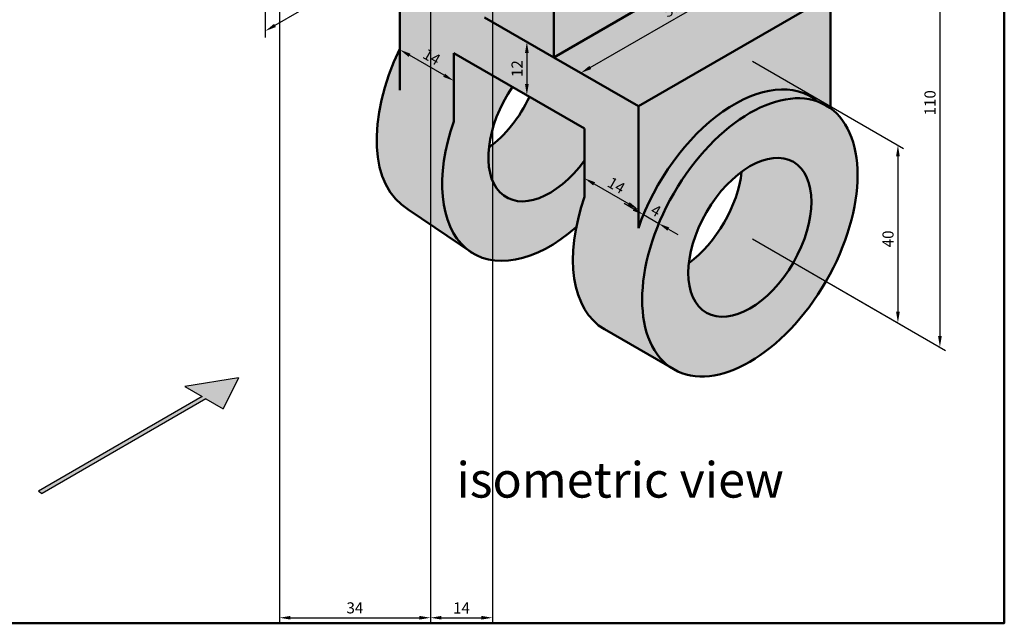
# Model space of a CAD drawing. Units: millimetres. Extents: x 1466 to 1886, y 5011 to 5605.
# Tile 2 of 4: x 1665 to 1886, y 5011 to 5146. Entities that reach past the tile are written whole.
import ezdxf

# ---------------------------------------------------------------- set-up
doc = ezdxf.new("R2010")
doc.units = ezdxf.units.MM
for name, color, linetype, lineweight in [('M-ANNO-SYMB', 3, 'Continuous', 25), ('M-DIMS', 2, 'Continuous', 25), ('M-HATC', 252, 'Continuous', 18), ('M-OUTL', 7, 'Continuous', 50), ('M-TEXT', 7, 'Continuous', 25), ('M-TTLB', 7, 'Continuous', 50)]:
    doc.layers.add(name, color=color, linetype=linetype, lineweight=lineweight)
doc.styles.get("Standard").update_dxf_attribs({"font": 'arial.ttf'})
doc.dimstyles.new('ISO-25', dxfattribs={"dimtxt": 2.5, "dimasz": 2.5, "dimexe": 1.25, "dimexo": 0.625, "dimtad": 1, "dimtxsty": 'Standard', "dimcen": 2.5, "dimadec": 0, "dimazin": 0, "dimtfac": 1, "dimtmove": 0, "dimatfit": 3, "dimfxl": 1, "dimarcsym": 0})

# ---------------------------------------------------------------- blocks, each defined once
blk = doc.blocks.new('*D1')
at = {"layer": 'Defpoints', "color": 0, "transparency": 16777216}
for p in [(1828.098835256636, 5162.955036981139), (1834.164568784784, 5159.452984095829), (1784.797565067414, 5137.955036981139)]:
    blk.add_point(p, dxfattribs=at)
at = {"layer": 'M-DIMS', "color": 0, "lineweight": -2, "transparency": 16777216}
for p, q in [((1828.723835256636, 5162.594193062894), (1835.414568784784, 5158.731296259342)), ((1793.028362105023, 5135.702984095829), (1831.999505275323, 5158.202984095829)), ((1785.422565067414, 5137.594193062894), (1792.113298595562, 5133.731296259342))]:
    blk.add_line(p, q, dxfattribs=at)
at = {"layer": 'M-DIMS', "color": 0, "transparency": 16777216}
for points in [[(1831.79117194199, 5158.563828014073), (1832.207838608656, 5157.842140177587), (1834.164568784784, 5159.452984095829)], [(1792.82002877169, 5136.063828014073), (1793.236695438357, 5135.342140177587), (1790.863298595562, 5134.45298409583)]]:
    blk.add_solid(points, dxfattribs=at)
at = {"layer": 'M-DIMS', "color": 0, "transparency": 16777216, "insert": (1811.563217455521, 5148.599672917828), "char_height": 2.5, "attachment_point": 5, "rotation": 30.000000000000025}
blk.add_mtext('50', dxfattribs=at)
blk = doc.blocks.new('*D11')
at = {"layer": 'Defpoints', "color": 0, "transparency": 16777216}
for p in [(1751.022574319821, 5185.455036981139), (1719.845659783581, 5167.455036981138), (1719.845659783581, 5143.908828507063)]:
    blk.add_point(p, dxfattribs=at)
at = {"layer": 'M-DIMS', "color": 0, "lineweight": -2, "transparency": 16777216}
for p, q in [((1751.022574319821, 5184.733349144652), (1751.022574319821, 5160.465452834088)), ((1719.845659783581, 5166.733349144652), (1719.845659783581, 5142.465452834088)), ((1748.85751081036, 5160.658828507063), (1722.010723293042, 5145.158828507063))]:
    blk.add_line(p, q, dxfattribs=at)
at = {"layer": 'M-DIMS', "color": 0, "transparency": 16777216}
for points in [[(1748.649177477027, 5161.019672425307), (1749.065844143693, 5160.297984588819), (1751.022574319821, 5161.908828507063)], [(1721.802389959709, 5145.519672425306), (1722.219056626375, 5144.797984588819), (1719.845659783581, 5143.908828507063)]]:
    blk.add_solid(points, dxfattribs=at)
at = {"layer": 'M-DIMS', "color": 0, "transparency": 16777216, "insert": (1734.482974486899, 5154.556255754542), "char_height": 2.5, "attachment_point": 5, "rotation": 30.00000000000017}
blk.add_mtext('36', dxfattribs=at)
blk = doc.blocks.new('*D13')
at = {"layer": 'Defpoints', "color": 0, "transparency": 16777216}
for p in [(1828.964860660421, 5137.45503698114), (1828.964860660421, 5097.45503698114), (1862.304605084383, 5078.206326563252)]:
    blk.add_point(p, dxfattribs=at)
at = {"layer": 'M-DIMS', "color": 0, "lineweight": -2, "transparency": 16777216}
for p, q in [((1829.589860660421, 5137.094193062897), (1863.554605084383, 5117.484638726765)), ((1862.304605084383, 5115.706326563252), (1862.304605084383, 5080.706326563252)), ((1829.589860660421, 5097.094193062897), (1863.554605084383, 5077.484638726765))]:
    blk.add_line(p, q, dxfattribs=at)
at = {"layer": 'M-DIMS', "color": 0, "transparency": 16777216}
for points in [[(1861.887938417716, 5115.706326563252), (1862.72127175105, 5115.706326563252), (1862.304605084383, 5118.206326563252)], [(1861.887938417716, 5080.706326563252), (1862.72127175105, 5080.706326563252), (1862.304605084383, 5078.206326563252)]]:
    blk.add_solid(points, dxfattribs=at)
at = {"layer": 'M-DIMS', "color": 0, "transparency": 16777216, "insert": (1860.40317261508, 5097.108534015251), "char_height": 2.5, "attachment_point": 5, "rotation": 90}
blk.add_mtext('40', dxfattribs=at)
blk = doc.blocks.new('*D14')
at = {"layer": 'Defpoints', "color": 0, "transparency": 16777216}
for p in [(1828.964860660421, 5207.455036981141), (1828.964860660421, 5097.45503698114), (1871.761163806512, 5072.74657983943)]:
    blk.add_point(p, dxfattribs=at)
at = {"layer": 'M-DIMS', "color": 0, "lineweight": -2, "transparency": 16777216}
for p, q in [((1829.589860660421, 5207.094193062896), (1873.011163806512, 5182.024892002942)), ((1871.761163806512, 5180.24657983943), (1871.761163806512, 5075.246579839429)), ((1829.589860660421, 5097.094193062897), (1873.011163806512, 5072.024892002943))]:
    blk.add_line(p, q, dxfattribs=at)
at = {"layer": 'M-DIMS', "color": 0, "transparency": 16777216}
for points in [[(1871.344497139845, 5180.24657983943), (1872.177830473179, 5180.24657983943), (1871.761163806512, 5182.74657983943)], [(1871.344497139845, 5075.246579839429), (1872.177830473179, 5075.246579839429), (1871.761163806512, 5072.74657983943)]]:
    blk.add_solid(points, dxfattribs=at)
at = {"layer": 'M-DIMS', "color": 0, "transparency": 16777216, "insert": (1869.859731337209, 5127.746579839429), "char_height": 2.5, "attachment_point": 5, "rotation": 90}
blk.add_mtext('110', dxfattribs=at)
blk = doc.blocks.new('*D15')
at = {"layer": 'Defpoints', "color": 0, "transparency": 16777216}
for p in [(1791.725768297689, 5106.564557194057), (1803.850123950672, 5103.757547358151), (1803.850123950672, 5099.564557194057)]:
    blk.add_point(p, dxfattribs=at)
at = {"layer": 'M-DIMS', "color": 0, "lineweight": -2, "transparency": 16777216}
for p, q in [((1791.725768297689, 5107.286245030543), (1791.725768297689, 5112.200923031124)), ((1793.890831807151, 5109.507547358151), (1801.68506044121, 5105.007547358151)), ((1803.850123950672, 5100.286245030543), (1803.850123950672, 5105.200923031125))]:
    blk.add_line(p, q, dxfattribs=at)
at = {"layer": 'M-DIMS', "color": 0, "transparency": 16777216}
for points in [[(1794.099165140484, 5109.868391276394), (1793.682498473817, 5109.146703439907), (1791.725768297689, 5110.757547358151)], [(1801.893393774544, 5105.368391276394), (1801.476727107877, 5104.646703439907), (1803.850123950672, 5103.757547358151)]]:
    blk.add_solid(points, dxfattribs=at)
at = {"layer": 'M-DIMS', "color": 0, "transparency": 16777216, "insert": (1798.728004105081, 5108.885775543131), "char_height": 2.5, "attachment_point": 5, "rotation": 329.99999999999994}
blk.add_mtext('14', dxfattribs=at)
blk = doc.blocks.new('*D16')
at = {"layer": 'Defpoints', "color": 0, "transparency": 16777216}
for p in [(1808.444159291447, 5100.569260893242), (1803.850123950671, 5099.564557194057), (1807.314225565809, 5097.564557194058)]:
    blk.add_point(p, dxfattribs=at)
at = {"layer": 'M-DIMS', "color": 0, "lineweight": -2, "transparency": 16777216}
for p, q in [((1802.814994166849, 5103.819260893242), (1800.649930657388, 5105.069260893242)), ((1804.073105504037, 5100.157506570685), (1805.42602078304, 5103.755159646497)), ((1804.98005767631, 5102.569260893242), (1808.444159291447, 5100.569260893242)), ((1807.537207119174, 5098.157506570685), (1808.890122398178, 5101.755159646497)), ((1810.609222800908, 5099.319260893242), (1812.774286310369, 5098.069260893242))]:
    blk.add_line(p, q, dxfattribs=at)
at = {"layer": 'M-DIMS', "color": 0, "transparency": 16777216}
for points in [[(1803.023327500182, 5104.180104811486), (1802.606660833515, 5103.458416974999), (1804.98005767631, 5102.569260893242)], [(1810.817556134242, 5099.680104811486), (1810.400889467575, 5098.958416974999), (1808.444159291447, 5100.569260893242)]]:
    blk.add_solid(points, dxfattribs=at)
at = {"layer": 'M-DIMS', "color": 0, "transparency": 16777216, "insert": (1807.649608483879, 5103.193058525338), "char_height": 2.5, "attachment_point": 5, "rotation": 329.99999999999784}
blk.add_mtext('4', dxfattribs=at)
blk = doc.blocks.new('*D17')
at = {"layer": 'Defpoints', "color": 0, "transparency": 16777216}
for p in [(1750.156548916035, 5145.955036981138), (1750.156548916035, 5139.692802544766), (1762.280904569018, 5138.955036981139)]:
    blk.add_point(p, dxfattribs=at)
at = {"layer": 'M-DIMS', "color": 0, "lineweight": -2, "transparency": 16777216}
for p, q in [((1750.156548916035, 5145.233349144651), (1750.156548916035, 5138.249426871792)), ((1760.115841059556, 5133.942802544765), (1752.321612425496, 5138.442802544766)), ((1762.280904569018, 5138.233349144652), (1762.280904569018, 5131.249426871792))]:
    blk.add_line(p, q, dxfattribs=at)
at = {"layer": 'M-DIMS', "color": 0, "transparency": 16777216}
for points in [[(1752.52994575883, 5138.80364646301), (1752.113279092163, 5138.081958626521), (1750.156548916035, 5139.692802544766)], [(1760.32417439289, 5134.30364646301), (1759.907507726223, 5133.581958626521), (1762.280904569018, 5132.692802544767)]]:
    blk.add_solid(points, dxfattribs=at)
at = {"layer": 'M-DIMS', "color": 0, "transparency": 16777216, "insert": (1757.158784723427, 5137.821030729746), "char_height": 2.5, "attachment_point": 5, "rotation": 329.9999999999995}
blk.add_mtext('14', dxfattribs=at)
blk = doc.blocks.new('*D23')
at = {"layer": 'Defpoints', "color": 0, "transparency": 16777216}
for p in [(1777.003336433355, 5142.45503698114), (1777.003336433355, 5130.455036981141), (1778.745424633516, 5129.449241889825)]:
    blk.add_point(p, dxfattribs=at)
at = {"layer": 'M-DIMS', "color": 0, "lineweight": -2, "transparency": 16777216}
for p, q in [((1777.628336433355, 5142.094193062897), (1779.995424633516, 5140.727554053338)), ((1778.745424633516, 5138.949241889825), (1778.745424633516, 5131.949241889826)), ((1777.628336433355, 5130.094193062897), (1779.995424633516, 5128.727554053338))]:
    blk.add_line(p, q, dxfattribs=at)
at = {"layer": 'M-DIMS', "color": 0, "transparency": 16777216}
for points in [[(1778.328757966849, 5138.949241889825), (1779.162091300183, 5138.949241889825), (1778.745424633516, 5141.449241889826)], [(1778.328757966849, 5131.949241889826), (1779.162091300183, 5131.949241889826), (1778.745424633516, 5129.449241889825)]]:
    blk.add_solid(points, dxfattribs=at)
at = {"layer": 'M-DIMS', "color": 0, "transparency": 16777216, "insert": (1776.865308671716, 5135.449241889824), "char_height": 2.5, "attachment_point": 5, "rotation": 90}
blk.add_mtext('12', dxfattribs=at)
blk = doc.blocks.new('*D57')
at = {"layer": 'Defpoints', "color": 0, "transparency": 16777216}
for p in [(1723.014464, 5426.716336000001), (1757.014464, 5426.716336000001), (1757.014464, 5011.829342)]:
    blk.add_point(p, dxfattribs=at)
at = {"layer": 'M-DIMS', "color": 0, "lineweight": -2, "transparency": 16777216}
for p, q in [((1723.014464, 5426.091336), (1723.014464, 5010.579341999999)), ((1757.014464, 5426.091336), (1757.014464, 5010.579341999999)), ((1725.514464, 5011.829342), (1754.514464, 5011.829342))]:
    blk.add_line(p, q, dxfattribs=at)
at = {"layer": 'M-DIMS', "color": 0, "transparency": 16777216}
for points in [[(1725.514464, 5012.246008666667), (1725.514464, 5011.412675333333), (1723.014464, 5011.829342)], [(1754.514464, 5012.246008666667), (1754.514464, 5011.412675333333), (1757.014464, 5011.829342)]]:
    blk.add_solid(points, dxfattribs=at)
at = {"layer": 'M-DIMS', "color": 0, "transparency": 16777216, "insert": (1740.014464, 5013.731627129605), "char_height": 2.5, "attachment_point": 5}
blk.add_mtext('34', dxfattribs=at)
blk = doc.blocks.new('*D58')
at = {"layer": 'Defpoints', "color": 0, "transparency": 16777216}
for p in [(1757.014464, 5426.716336000001), (1771.014464, 5426.716336000001), (1771.014464, 5011.829342)]:
    blk.add_point(p, dxfattribs=at)
at = {"layer": 'M-DIMS', "color": 0, "lineweight": -2, "transparency": 16777216}
for p, q in [((1757.014464, 5426.091336), (1757.014464, 5010.579341999999)), ((1771.014464, 5426.091336), (1771.014464, 5010.579341999999)), ((1759.514464, 5011.829342), (1768.514464, 5011.829342))]:
    blk.add_line(p, q, dxfattribs=at)
at = {"layer": 'M-DIMS', "color": 0, "transparency": 16777216}
for points in [[(1759.514464, 5012.246008666667), (1759.514464, 5011.412675333333), (1757.014464, 5011.829342)], [(1768.514464, 5012.246008666667), (1768.514464, 5011.412675333333), (1771.014464, 5011.829342)]]:
    blk.add_solid(points, dxfattribs=at)
at = {"layer": 'M-DIMS', "color": 0, "transparency": 16777216, "insert": (1764.014464, 5013.709457961801), "char_height": 2.5, "attachment_point": 5}
blk.add_mtext('14', dxfattribs=at)

msp = doc.modelspace()

# ---------------------------------------------------------------- hatches: boundary and pattern name
at = {"layer": 'M-ANNO-SYMB'}
h = msp.add_hatch(color=256, dxfattribs=at)
h.dxf.hatch_style = 1
h.paths.add_polyline_path([(1706.476050365284, 5061.122786737217), (1710.373164682314, 5058.872786737217), (1713.837266297452, 5065.872786737217), (1701.71291064447, 5063.872786737217), (1705.6100249615, 5061.622786737217), (1668.728696067036, 5040.329341571927), (1669.59472147082, 5039.829341571927)])
at = {"layer": 'M-HATC'}
h = msp.add_hatch(color=256, dxfattribs=at)
h.dxf.hatch_style = 1
edge = h.paths.add_edge_path()
edge.add_line((1722.443735994935, 5219.955036981139), (1738.032193263055, 5210.955036981139))
edge.add_line((1738.032193263055, 5210.955036981139), (1722.443735994935, 5201.955036981138))
edge.add_line((1722.443735994935, 5201.955036981138), (1732.836040840348, 5195.955036981139))
edge.add_line((1732.836040840348, 5195.955036981139), (1758.816802953881, 5210.955036981139))
edge.add_line((1758.816802953881, 5210.955036981139), (1748.424498108468, 5216.955036981139))
edge.add_line((1748.424498108468, 5216.955036981139), (1732.836040840348, 5225.955036981138))
edge.add_line((1732.836040840348, 5225.955036981138), (1722.443735994935, 5231.955036981139))
edge.add_line((1722.443735994935, 5231.955036981139), (1712.051431149521, 5225.955036981138))
edge.add_line((1712.051431149521, 5225.955036981138), (1702.481741639855, 5220.429974166671))
edge.add_ellipse((1693.864897670048, 5200.455036981139), major_axis=(-11.02270384252446, -19.0918830920367), ratio=0.5773502691896324, start_angle=186.6654644117269, end_angle=360)
edge.add_line((1682.842193827524, 5181.363153889102), (1695.83257488429, 5173.863153889102))
edge.add_ellipse((1706.855278726814, 5192.955036981139), major_axis=(-11.02270384252446, -19.09188309203669), ratio=0.5773502691896325, start_angle=270, end_angle=359.9999999999998, ccw=False)
edge.add_ellipse((1706.855278726814, 5192.955036981139), major_axis=(-11.02270384252446, -19.09188309203669), ratio=0.5773502691896325, start_angle=210.0000000000012, end_angle=270, ccw=False)
edge.add_line((1706.855278726813, 5210.955036981138), (1722.443735994935, 5219.955036981139))
edge = h.paths.add_edge_path(flags=17)
edge.add_ellipse((1735.434117051701, 5176.455036981138), major_axis=(-11.02270384252446, -19.0918830920367), ratio=0.5773502691896324, start_angle=183.919715644874, end_angle=270, ccw=False)
edge.add_ellipse((1732.836040840348, 5177.955036981138), major_axis=(-11.02270384252446, -19.0918830920367), ratio=0.5773502691896323, start_angle=176.0802843551266, end_angle=210.0000000000004)
edge.add_line((1732.836040840348, 5195.955036981139), (1722.443735994935, 5201.955036981138))
edge.add_ellipse((1722.443735994935, 5183.955036981139), major_axis=(-11.02270384252446, -19.0918830920367), ratio=0.5773502691896323, start_angle=210.0000000000004, end_angle=266.235889459397)
edge.add_ellipse((1706.855278726814, 5192.955036981139), major_axis=(-4.592793267718468, -7.954951288348655), ratio=0.5773502691896232, start_angle=90, end_angle=99.00326933995552, ccw=False)
edge.add_line((1711.448071994533, 5190.303386551689), (1724.411413209177, 5182.818998011818))
edge = h.paths.add_edge_path()
edge.add_line((1724.411413209177, 5182.818998011818), (1711.448071994533, 5190.303386551689))
edge.add_ellipse((1706.855278726814, 5192.955036981139), major_axis=(-4.592793267718468, -7.954951288348655), ratio=0.5773502691896232, start_angle=80.9967306600526, end_angle=90, ccw=False)
edge.add_ellipse((1722.443735994935, 5183.955036981139), major_axis=(-11.02270384252446, -19.0918830920367), ratio=0.5773502691896323, start_angle=273.764110540599, end_angle=329.9999999999981)
edge.add_ellipse((1722.443735994935, 5183.955036981139), major_axis=(-11.02270384252446, -19.0918830920367), ratio=0.5773502691896323, start_angle=329.9999999999981, end_angle=360)
edge.add_line((1711.42103215241, 5164.863153889102), (1724.411413209177, 5157.363153889102))
edge.add_ellipse((1735.434117051701, 5176.455036981138), major_axis=(-11.02270384252446, -19.0918830920367), ratio=0.5773502691896324, start_angle=270, end_angle=360, ccw=False)
edge = h.paths.add_edge_path(flags=17)
edge.add_line((1758.816802953881, 5210.955036981139), (1732.836040840348, 5195.955036981139))
edge.add_ellipse((1732.836040840348, 5177.955036981138), major_axis=(-11.02270384252446, -19.0918830920367), ratio=0.5773502691896323, start_angle=176.0802843551266, end_angle=210.0000000000005, ccw=False)
edge.add_ellipse((1735.434117051701, 5176.455036981138), major_axis=(-11.02270384252446, -19.0918830920367), ratio=0.5773502691896324, start_angle=70.6800531201103, end_angle=183.919715644874, ccw=False)
edge.add_line((1744.050961021509, 5166.429974166671), (1758.816802953881, 5174.955036981138))
edge.add_line((1758.816802953881, 5174.955036981138), (1758.816802953881, 5210.955036981139))
edge = h.paths.add_edge_path(flags=17)
edge.add_ellipse((1797.78794612418, 5225.455036981139), major_axis=(-15.30931089239438, -26.5165042944958), ratio=0.5773502691896226, start_angle=218.6849191088683, end_angle=329.99999999999915, ccw=False)
edge.add_line((1794.323844509042, 5248.132962339644), (1748.424498108468, 5216.955036981139))
edge.add_line((1748.424498108468, 5216.955036981139), (1758.816802953881, 5210.955036981139))
edge.add_line((1758.816802953881, 5210.955036981139), (1758.816802953881, 5186.955036981139))
edge.add_line((1758.816802953881, 5186.955036981139), (1776.13731102957, 5196.955036981139))
edge.add_line((1776.13731102957, 5196.955036981139), (1776.13731102957, 5212.955036981139))
edge = h.paths.add_edge_path()
edge.add_ellipse((1797.78794612418, 5225.455036981139), major_axis=(-15.30931089239438, -26.5165042944958), ratio=0.5773502691896226, start_angle=218.6849191088682, end_angle=329.9999999999991)
edge.add_line((1776.13731102957, 5212.955036981139), (1776.13731102957, 5196.955036981139))
edge.add_line((1776.13731102957, 5196.955036981139), (1769.209107799294, 5192.955036981139))
edge.add_line((1769.209107799294, 5192.955036981139), (1769.209107799294, 5146.955036981139))
edge.add_line((1769.209107799294, 5146.955036981139), (1784.797565067414, 5137.955036981139))
edge.add_line((1784.797565067414, 5137.955036981139), (1784.797565067414, 5155.95503698114))
edge.add_line((1784.797565067414, 5155.95503698114), (1784.797565067414, 5207.955036981145))
edge.add_ellipse((1806.448200162025, 5220.455036981139), major_axis=(-15.30931089239438, -26.5165042944958), ratio=0.5773502691896227, start_angle=329.9999999999989, end_angle=363.7613167964908)
edge.add_ellipse((1809.912301777163, 5218.455036981139), major_axis=(-15.30931089239438, -26.5165042944958), ratio=0.5773502691896226, start_angle=179.9999999999992, end_angle=356.23868320351306, ccw=False)
edge.add_line((1825.221612669557, 5244.971541275634), (1785.384444095473, 5267.971541275635))
edge.add_ellipse((1770.075133203079, 5241.455036981139), major_axis=(-15.30931089239438, -26.5165042944958), ratio=0.5773502691896226, start_angle=540, end_angle=311.5164128123438)
edge.add_line((1749.475859885243, 5237.257922029503), (1732.836040840348, 5225.955036981138))
edge.add_line((1732.836040840348, 5225.955036981138), (1748.424498108468, 5216.955036981139))
edge.add_line((1748.424498108468, 5216.955036981139), (1794.323844509042, 5248.132962339644))
edge = h.paths.add_edge_path()
edge.add_line((1828.098835256636, 5207.955036981139), (1825.221612669557, 5209.616202216307))
edge.add_ellipse((1809.912301777163, 5218.455036981139), major_axis=(-15.30931089239438, -26.5165042944958), ratio=0.5773502691896226, start_angle=356.23868320351306, end_angle=449.99999999999966, ccw=False)
edge.add_ellipse((1806.448200162025, 5220.455036981139), major_axis=(-15.30931089239438, -26.5165042944958), ratio=0.5773502691896227, start_angle=329.99999999999886, end_angle=363.76131679649075, ccw=False)
edge.add_line((1784.797565067414, 5207.955036981145), (1784.797565067414, 5155.95503698114))
edge.add_line((1784.797565067414, 5155.95503698114), (1784.797565067414, 5137.955036981139))
edge.add_line((1784.797565067414, 5137.955036981139), (1828.098835256636, 5162.955036981139))
edge.add_line((1828.098835256636, 5162.955036981139), (1828.098835256636, 5207.955036981139))
edge = h.paths.add_edge_path()
edge.add_ellipse((1809.912301777163, 5218.455036981139), major_axis=(-15.30931089239438, -26.5165042944958), ratio=0.5773502691896226, start_angle=89.99999999999972, end_angle=110.43480323036249, ccw=False)
edge.add_line((1825.221612669557, 5209.616202216307), (1828.098835256636, 5207.955036981139))
edge.add_line((1828.098835256636, 5207.955036981139), (1828.098835256636, 5215.390377014889))
h.paths.add_polyline_path([(1769.209107799294, 5168.955036981138), (1750.156548916036, 5157.955036981139), (1769.209107799294, 5146.955036981139)], flags=17)
h.paths.add_polyline_path([(1847.151394139893, 5151.955036981139), (1828.098835256636, 5162.955036981139), (1784.797565067414, 5137.955036981139), (1803.850123950671, 5126.955036981138)])
edge = h.paths.add_edge_path()
edge.add_ellipse((1825.500759045282, 5099.455036981138), major_axis=(-17.14642819948207, -29.69848480983509), ratio=0.577350269189623, start_angle=176.6451013603207, end_angle=299.71017051362753, ccw=False)
edge.add_ellipse((1828.96486066042, 5097.455036981139), major_axis=(-17.14642819948207, -29.69848480983509), ratio=0.577350269189623, start_angle=177.9252840891673, end_angle=183.3548986396804, ccw=False)
edge.add_line((1847.151394139893, 5126.47529615859), (1847.151394139893, 5151.955036981139))
edge.add_line((1847.151394139893, 5151.955036981139), (1804.3764033923, 5127.258884558432))
edge.add_ellipse((1813.3764033923, 5106.455036981138), major_axis=(-17.14642819948207, -29.69848480983509), ratio=0.577350269189623, start_angle=233.3939017938641, end_angle=235.1951901217888)
edge.add_line((1803.850123950671, 5126.703823360306), (1803.850123950671, 5099.564557194057))
edge = h.paths.add_edge_path()
edge.add_ellipse((1828.96486066042, 5097.455036981139), major_axis=(-17.14642819948207, -29.69848480983509), ratio=0.577350269189623, start_angle=183.3548986396804, end_angle=360, ccw=False)
edge.add_ellipse((1825.500759045282, 5099.455036981138), major_axis=(-17.14642819948207, -29.69848480983509), ratio=0.577350269189623, start_angle=176.6451013603206, end_angle=299.7101705136275)
edge.add_line((1803.850123950671, 5099.564557194057), (1803.850123950671, 5126.703823360306))
edge.add_line((1803.850123950671, 5126.703823360306), (1803.850123950671, 5126.955036981138))
edge.add_line((1803.850123950671, 5126.955036981138), (1784.797565067414, 5137.955036981139))
edge.add_line((1784.797565067414, 5137.955036981139), (1769.209107799294, 5146.955036981139))
edge.add_line((1769.209107799294, 5146.955036981139), (1750.156548916036, 5157.955036981139))
edge.add_line((1750.156548916036, 5157.955036981139), (1750.156548916036, 5139.867928007788))
edge.add_ellipse((1769.165624306577, 5133.458728431643), major_axis=(-17.14642819948207, -29.69848480983509), ratio=0.577350269189623, start_angle=281.3676816797435, end_angle=360)
edge.add_line((1752.019196107095, 5103.760243621808), (1765.421555363387, 5094.680341464254))
edge.add_ellipse((1783.931539663629, 5123.455036981138), major_axis=(-17.14642819948207, -29.69848480983509), ratio=0.577350269189623, start_angle=299.7101705136324, end_angle=357.2479180547133, ccw=False)
edge.add_line((1762.280904569018, 5123.564557194055), (1762.280904569018, 5138.955036981139))
edge.add_line((1762.280904569018, 5138.955036981139), (1784.797565067414, 5125.955036981139))
edge.add_line((1784.797565067414, 5125.955036981139), (1791.725768297689, 5121.955036981138))
edge.add_line((1791.725768297689, 5121.955036981138), (1791.725768297689, 5106.564557194055))
edge.add_ellipse((1813.3764033923, 5106.455036981138), major_axis=(-17.14642819948207, -29.69848480983509), ratio=0.577350269189623, start_angle=299.7101705136277, end_angle=315.9583021122638)
edge.add_ellipse((1813.3764033923, 5106.455036981138), major_axis=(-17.14642819948207, -29.69848480983509), ratio=0.577350269189623, start_angle=315.9583021122638, end_angle=360)
edge.add_line((1796.229975192818, 5076.756552171303), (1811.818432460938, 5067.756552171303))
h = msp.add_hatch(color=256, dxfattribs=at)
h.dxf.hatch_style = 1
edge = h.paths.add_edge_path()
edge.add_ellipse((1809.912301777163, 5218.455036981139), major_axis=(-7.654655446197786, -13.25825214724756), ratio=0.5773502691896373, start_angle=90, end_angle=360, ccw=False)
edge.add_line((1817.56695722336, 5214.035619598722), (1825.221612669557, 5209.616202216307))
edge.add_ellipse((1809.912301777163, 5218.455036981139), major_axis=(-15.30931089239438, -26.5165042944958), ratio=0.5773502691896226, start_angle=89.99999999999962, end_angle=110.4348032303624)
edge.add_ellipse((1809.912301777163, 5218.455036981139), major_axis=(-15.30931089239438, -26.5165042944958), ratio=0.5773502691896226, start_angle=110.4348032303624, end_angle=179.9999999999991)
edge.add_ellipse((1809.912301777163, 5218.455036981139), major_axis=(-15.30931089239438, -26.5165042944958), ratio=0.5773502691896226, start_angle=179.9999999999991, end_angle=356.2386832035131)
edge.add_ellipse((1809.912301777163, 5218.455036981139), major_axis=(-15.30931089239438, -26.5165042944958), ratio=0.5773502691896226, start_angle=356.2386832035131, end_angle=449.9999999999996)
edge.add_line((1825.221612669557, 5209.616202216307), (1817.56695722336, 5214.035619598722))
edge.add_ellipse((1809.912301777163, 5218.455036981139), major_axis=(-7.654655446197786, -13.25825214724756), ratio=0.5773502691896373, start_angle=0, end_angle=90, ccw=False)
edge = h.paths.add_edge_path()
edge.add_ellipse((1735.434117051701, 5176.455036981138), major_axis=(-11.02270384252446, -19.0918830920367), ratio=0.5773502691896324, start_angle=70.68005312011024, end_angle=183.9197156448739)
edge.add_ellipse((1735.434117051701, 5176.455036981138), major_axis=(-11.02270384252446, -19.0918830920367), ratio=0.5773502691896324, start_angle=183.9197156448739, end_angle=270)
edge.add_line((1724.411413209177, 5182.818998011818), (1730.841323783983, 5179.106687410587))
edge.add_ellipse((1735.434117051701, 5176.455036981138), major_axis=(-4.592793267718468, -7.954951288348655), ratio=0.5773502691896234, start_angle=0, end_angle=270, ccw=False)
edge.add_ellipse((1735.434117051701, 5176.455036981138), major_axis=(-4.592793267718468, -7.954951288348655), ratio=0.5773502691896234, start_angle=270, end_angle=360, ccw=False)
edge.add_line((1730.841323783983, 5179.106687410587), (1724.411413209177, 5182.818998011818))
edge.add_ellipse((1735.434117051701, 5176.455036981138), major_axis=(-11.02270384252446, -19.0918830920367), ratio=0.5773502691896324, start_angle=270, end_angle=360)
edge.add_ellipse((1735.434117051701, 5176.455036981138), major_axis=(-11.02270384252446, -19.0918830920367), ratio=0.5773502691896324, start_angle=0, end_angle=70.68005312011029)
edge = h.paths.add_edge_path()
edge.add_line((1722.443735994935, 5219.955036981139), (1706.855278726813, 5210.955036981138))
edge.add_ellipse((1706.855278726814, 5192.955036981139), major_axis=(-11.02270384252446, -19.09188309203669), ratio=0.5773502691896325, start_angle=210.0000000000012, end_angle=270)
edge.add_line((1695.83257488429, 5199.318998011818), (1702.262485459096, 5195.606687410588))
edge.add_ellipse((1706.855278726814, 5192.955036981139), major_axis=(-4.592793267718468, -7.954951288348655), ratio=0.5773502691896232, start_angle=99.00326933995552, end_angle=270, ccw=False)
edge.add_ellipse((1722.443735994935, 5183.955036981139), major_axis=(-11.02270384252446, -19.0918830920367), ratio=0.5773502691896323, start_angle=210.0000000000005, end_angle=266.2358894593971, ccw=False)
edge.add_line((1722.443735994935, 5201.955036981138), (1722.443735994935, 5219.955036981139))
edge = h.paths.add_edge_path()
edge.add_ellipse((1722.443735994935, 5183.955036981139), major_axis=(-11.02270384252446, -19.0918830920367), ratio=0.5773502691896323, start_angle=273.76411054059906, end_angle=329.9999999999982, ccw=False)
edge.add_ellipse((1706.855278726814, 5192.955036981139), major_axis=(-4.592793267718468, -7.954951288348655), ratio=0.5773502691896232, start_angle=270, end_angle=440.9967306600526, ccw=False)
edge.add_line((1702.262485459096, 5195.606687410588), (1695.83257488429, 5199.318998011818))
edge.add_ellipse((1706.855278726814, 5192.955036981139), major_axis=(-11.02270384252446, -19.09188309203669), ratio=0.5773502691896325, start_angle=270, end_angle=359.9999999999997)
edge.add_ellipse((1706.855278726814, 5192.955036981139), major_axis=(-11.02270384252446, -19.09188309203669), ratio=0.5773502691896325, start_angle=359.9999999999997, end_angle=390.0000000000012)
edge = h.paths.add_edge_path()
edge.add_ellipse((1828.96486066042, 5097.455036981139), major_axis=(-17.14642819948207, -29.69848480983509), ratio=0.577350269189623, start_angle=0, end_angle=177.9252840891672)
edge.add_ellipse((1828.96486066042, 5097.455036981139), major_axis=(-17.14642819948207, -29.69848480983509), ratio=0.577350269189623, start_angle=177.9252840891672, end_angle=183.3548986396804)
edge.add_ellipse((1828.96486066042, 5097.455036981139), major_axis=(-17.14642819948207, -29.69848480983509), ratio=0.577350269189623, start_angle=183.3548986396804, end_angle=360)
edge = h.paths.add_edge_path(flags=16)
edge.add_ellipse((1828.96486066042, 5097.455036981139), major_axis=(-9.79795897113284, -16.97056274847708), ratio=0.5773502691896234, start_angle=217.1598249325803, end_angle=322.84017506741907, ccw=False)
edge.add_ellipse((1828.96486066042, 5097.455036981139), major_axis=(-9.79795897113284, -16.97056274847708), ratio=0.5773502691896234, start_angle=322.84017506741907, end_angle=577.1598249325802, ccw=False)
edge = h.paths.add_edge_path()
edge.add_line((1791.725768297689, 5106.564557194055), (1791.725768297689, 5114.726280425816))
edge.add_ellipse((1783.931539663629, 5123.455036981138), major_axis=(-9.797958971132836, -16.97056274847707), ratio=0.5773502691896235, start_angle=322.84017506742066, end_angle=431.7628416390562, ccw=False)
edge.add_ellipse((1783.931539663629, 5123.455036981138), major_axis=(-9.797958971132836, -16.97056274847707), ratio=0.5773502691896235, start_angle=256.9555772654587, end_angle=322.84017506742066, ccw=False)
edge.add_line((1775.519115469529, 5131.31195235414), (1762.280904569018, 5138.955036981139))
edge.add_line((1762.280904569018, 5138.955036981139), (1762.280904569018, 5123.564557194055))
edge.add_ellipse((1783.931539663629, 5123.455036981138), major_axis=(-17.14642819948207, -29.69848480983509), ratio=0.577350269189623, start_angle=299.7101705136324, end_angle=357.2479180547133)
edge.add_line((1765.421555363387, 5094.680341464254), (1766.785111464145, 5093.756552171305))
edge.add_ellipse((1783.931539663629, 5123.455036981138), major_axis=(-17.14642819948207, -29.69848480983509), ratio=0.577350269189623, start_angle=359.9999999999943, end_angle=404.0416978877337)
edge.add_ellipse((1813.3764033923, 5106.455036981138), major_axis=(-17.14642819948207, -29.69848480983509), ratio=0.577350269189623, start_angle=299.71017051362776, end_angle=315.95830211226377, ccw=False)
h = msp.add_hatch(color=256, dxfattribs=at)
h.dxf.hatch_style = 1
edge = h.paths.add_edge_path()
edge.add_ellipse((1735.434117051701, 5176.455036981138), major_axis=(-4.592793267718468, -7.954951288348655), ratio=0.5773502691896234, start_angle=0, end_angle=270)
edge.add_ellipse((1735.434117051701, 5176.455036981138), major_axis=(-4.592793267718468, -7.954951288348655), ratio=0.5773502691896234, start_angle=270, end_angle=360)
edge = h.paths.add_edge_path()
edge.add_ellipse((1809.912301777163, 5218.455036981139), major_axis=(-7.654655446197786, -13.25825214724756), ratio=0.5773502691896373, start_angle=90.00000000000003, end_angle=360)
edge.add_ellipse((1809.912301777163, 5218.455036981139), major_axis=(-7.654655446197786, -13.25825214724756), ratio=0.5773502691896373, start_angle=0, end_angle=90)
edge = h.paths.add_edge_path()
edge.add_ellipse((1706.855278726814, 5192.955036981139), major_axis=(-4.592793267718468, -7.954951288348655), ratio=0.5773502691896232, start_angle=99.00326933995547, end_angle=270)
edge.add_line((1702.262485459096, 5195.606687410588), (1711.42103215241, 5190.318998011818))
edge.add_ellipse((1722.443735994935, 5183.955036981139), major_axis=(-11.02270384252446, -19.0918830920367), ratio=0.5773502691896323, start_angle=266.2358894593971, end_angle=270, ccw=False)
edge = h.paths.add_edge_path()
edge.add_ellipse((1722.443735994935, 5183.955036981139), major_axis=(-11.02270384252446, -19.0918830920367), ratio=0.5773502691896323, start_angle=270, end_angle=273.76411054059906, ccw=False)
edge.add_line((1711.42103215241, 5190.318998011818), (1702.262485459096, 5195.606687410588))
edge.add_ellipse((1706.855278726814, 5192.955036981139), major_axis=(-4.592793267718468, -7.954951288348655), ratio=0.5773502691896232, start_angle=270, end_angle=440.9967306600525)
edge = h.paths.add_edge_path()
edge.add_ellipse((1828.96486066042, 5097.455036981139), major_axis=(-9.79795897113284, -16.97056274847708), ratio=0.5773502691896234, start_angle=322.840175067419, end_angle=217.1598249325803)
edge.add_ellipse((1813.3764033923, 5106.455036981138), major_axis=(-9.797958971132836, -16.97056274847707), ratio=0.5773502691896235, start_angle=397.1598249325802, end_angle=502.8401750674186, ccw=False)
edge = h.paths.add_edge_path()
edge.add_line((1791.725768297689, 5121.955036981138), (1784.797565067414, 5125.955036981139))
edge.add_line((1784.797565067414, 5125.955036981139), (1779.353582800964, 5129.098121608137))
edge.add_ellipse((1768.343082395509, 5132.455036981139), major_axis=(-9.797958971132836, -16.97056274847707), ratio=0.5773502691896235, start_angle=397.1598249325797, end_angle=463.0444227345428, ccw=False)
edge.add_ellipse((1783.931539663629, 5123.455036981138), major_axis=(-9.797958971132836, -16.97056274847707), ratio=0.5773502691896235, start_angle=322.8401750674207, end_angle=431.7628416390561)
edge.add_line((1791.725768297689, 5114.726280425816), (1791.725768297689, 5121.955036981138))

# ---------------------------------------------------------------- linework, layer by layer
at = {"layer": 'M-ANNO-SYMB'}
for p, q in [((1713.837266297452, 5065.872786737217), (1701.71291064447, 5063.872786737217)), ((1713.837266297452, 5065.872786737217), (1710.373164682314, 5058.872786737217)), ((1701.71291064447, 5063.872786737217), (1705.6100249615, 5061.622786737217)), ((1705.6100249615, 5061.622786737217), (1668.728696067036, 5040.329341571927)), ((1706.476050365284, 5061.122786737217), (1669.59472147082, 5039.829341571927)), ((1706.476050365284, 5061.122786737217), (1710.373164682314, 5058.872786737217)), ((1668.728696067036, 5040.329341571927), (1669.59472147082, 5039.829341571927))]:
    msp.add_line(p, q, dxfattribs=at)
at = {"layer": 'M-OUTL'}
for p, q in [((1784.797565067414, 5137.955036981139), (1828.098835256636, 5162.955036981139)), ((1750.156548916036, 5157.955036981139), (1750.156548916036, 5130.564557194056)), ((1784.797565067414, 5137.955036981139), (1784.797565067414, 5155.95503698114)), ((1847.151394139893, 5151.955036981139), (1803.850123950671, 5126.955036981138)), ((1847.151394139893, 5151.955036981139), (1847.151394139893, 5126.47529615859)), ((1784.797565067414, 5137.955036981139), (1769.209107799294, 5146.955036981139)), ((1784.797565067414, 5125.955036981139), (1762.280904569018, 5138.955036981139)), ((1762.280904569018, 5138.95503698114), (1762.280904569018, 5123.564557194057)), ((1803.850123950671, 5126.955036981138), (1784.797565067414, 5137.955036981139)), ((1769.209107799294, 5134.955036981139), (1768.133428884185, 5135.576080492338)), ((1803.850123950671, 5126.955036981138), (1803.850123950671, 5099.564557194057)), ((1791.725768297689, 5121.955036981138), (1784.797565067414, 5125.955036981139)), ((1791.725768297689, 5121.955036981138), (1791.725768297689, 5106.564557194057)), ((1766.785111464147, 5093.756552171303), (1752.019196107095, 5103.760243621808)), ((1811.818432460938, 5067.756552171303), (1796.229975192818, 5076.756552171303))]:
    msp.add_line(p, q, dxfattribs=at)
for centre, major_axis, ratio, start_param, end_param in [((1769.165624306577, 5133.458728431643), (-17.14642819948207, -29.69848480983509), 0.577350269189623, 4.827947213190288, 6.283185307179586), ((1783.931539663629, 5123.455036981138), (-9.797958971132834, -16.97056274847707), 0.5773502691896234, 4.57941492851331, 7.665989887222072), ((1825.500759045282, 5099.455036981138), (-17.14642819948207, -29.69848480983509), 0.577350269189623, 3.040404810806179, 5.030641032773306), ((1768.343082395509, 5132.455036981139), (-9.797958971132834, -16.97056274847707), 0.5773502691896234, 7.203009547241259, 7.986955685845877), ((1783.931539663629, 5123.455036981138), (-17.14642819948207, -29.69848480983509), 0.577350269189623, 5.030641032773365, 7.315775638405188), ((1813.3764033923, 5106.455036981138), (-9.797958971132834, -16.97056274847707), 0.5773502691896234, 7.203009547241268, 8.504953720707675), ((1813.3764033923, 5106.455036981138), (-17.14642819948207, -29.69848480983509), 0.577350269189623, 5.030641032773309, 6.283185307179586)]:
    msp.add_ellipse(centre, major_axis=major_axis, ratio=ratio, start_param=start_param, end_param=end_param, dxfattribs=at)
for major_axis, ratio in [((-17.14642819948207, -29.69848480983509), 0.577350269189623), ((-9.797958971132832, -16.97056274847707), 0.5773502691896234)]:
    msp.add_ellipse((1828.96486066042, 5097.455036981139), major_axis=major_axis, ratio=ratio, dxfattribs=at)
at = {"layer": 'M-TTLB'}
msp.add_lwpolyline([(1466.267100225985, 5604.631473972534), (1886.267100225985, 5604.631473972534), (1886.267100225985, 5010.631473972534), (1466.267100225985, 5010.631473972534)], close=True, dxfattribs=at)

# ---------------------------------------------------------------- texts
at = {"layer": 'M-TEXT', "insert": (1762.892180069171, 5046.869127239424), "char_height": 8, "attachment_point": 1}
msp.add_mtext_dynamic_manual_height_columns('isometric view', width=80.41530136712912, gutter_width=12.5, heights=[0], dxfattribs=at)

# ---------------------------------------------------------------- dimensions: what is measured, and where the dimension line sits
at = {"layer": 'M-DIMS'}
for base, p1, p2, picture, middle in [((1757.014464, 5011.829342), (1723.014464, 5426.716336000001), (1757.014464, 5426.716336000001), '*D57', (1740.014464, 5013.731627129605)), ((1771.014464, 5011.829342), (1757.014464, 5426.716336000001), (1771.014464, 5426.716336000001), '*D58', (1764.014464, 5013.709457961801))]:
    dim = msp.add_linear_dim(base=base, p1=p1, p2=p2, dimstyle='ISO-25', override={"dimdec": 0, "dimlfac": 1, "dimrnd": 0, "dimzin": 0, "dimdsep": 46, "dimlunit": 2}, dxfattribs=at)
    dim.commit()
    dim.dimension.update_dxf_attribs({"geometry": picture, "text_midpoint": middle})
for p1, p2, distance, picture, middle in [((1828.96486066042, 5207.455036981139), (1828.96486066042, 5097.455036981139), 42.79630314609198, '*D14', (1869.859731337209, 5127.746579839429)), ((1751.022574319821, 5185.455036981139), (1719.845659783581, 5167.455036981138), 20.391614701352964, '*D11', (1734.482974486899, 5154.556255754542)), ((1784.797565067414, 5137.955036981139), (1828.098835256636, 5162.955036981139), -6.065733528148409, '*D1', (1811.563217455521, 5148.599672917828)), ((1762.280904569018, 5138.955036981139), (1750.156548916036, 5145.955036981138), 5.4232541063522675, '*D17', (1757.158784723427, 5137.821030729746)), ((1777.003336433354, 5142.455036981139), (1777.003336433354, 5130.455036981139), 1.7420882001620157, '*D23', (1776.865308671716, 5135.449241889824)), ((1791.725768297689, 5106.564557194057), (1803.850123950671, 5099.564557194057), 3.631235999924334, '*D15', (1798.728004105081, 5108.885775543131)), ((1803.850123950671, 5099.564557194057), (1807.314225565809, 5097.564557194057), 3.1671165971587207, '*D16', (1807.649608483879, 5103.193058525338))]:
    dim = msp.add_aligned_dim(p1=p1, p2=p2, distance=distance, dimstyle='ISO-25', override={"dimclrd": 0, "dimclre": 0, "dimclrt": 0}, dxfattribs=at)
    dim.commit()
    dim.dimension.update_dxf_attribs({"geometry": picture, "text_midpoint": middle})
dim = msp.add_linear_dim(base=(1862.304605084383, 5078.206326563252), p1=(1828.96486066042, 5137.455036981139), p2=(1828.96486066042, 5097.455036981139), angle=270, dimstyle='ISO-25', override={"dimclrd": 0, "dimclre": 0, "dimclrt": 0}, dxfattribs=at)
dim.commit()
dim.dimension.update_dxf_attribs({"geometry": '*D13', "text_midpoint": (1862.304605084384, 5097.108534015251), "dimtype": 161})

doc.saveas('drawing.dxf')
